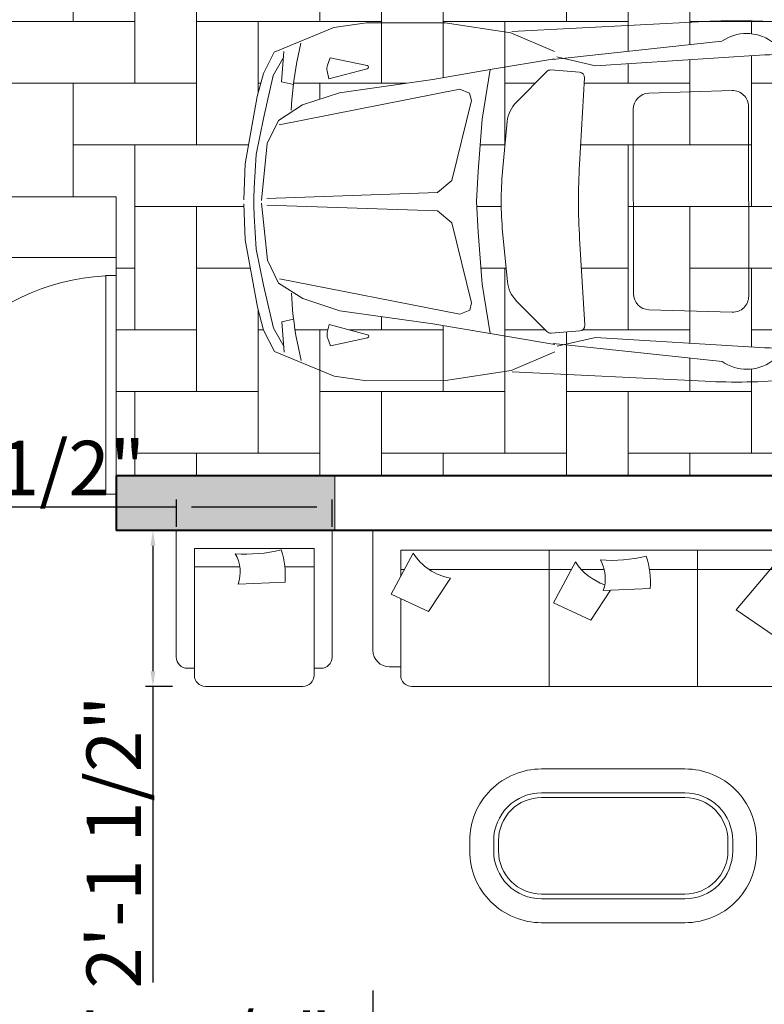
# Model space of a CAD drawing. Units: inches. Extents: x 2337 to 3570, y 1258 to 1938.
# Tile 13 of 30: x 2704 to 2827, y 1677 to 1839. Entities that reach past the tile are written whole.
import ezdxf

# ---------------------------------------------------------------- set-up
doc = ezdxf.new("R2010")
doc.units = ezdxf.units.IN
for name, color, linetype, lineweight in [('A-ANNO-DIMS', 2, 'Continuous', 18), ('A-DOOR', 4, 'Continuous', 20), ('A-FLOR-PATT', 252, 'Continuous', 13), ('A-FLOR-STRS', 7, 'Continuous', 20), ('A-GLAZ', 4, 'Continuous', 18), ('A-WALL', 7, 'Continuous', 40), ('furn', 8, 'Continuous', 18), ('L-SITE-VEHI', 8, 'Continuous', 18)]:
    doc.layers.add(name, color=color, linetype=linetype, lineweight=lineweight)
doc.layers.add('A-WALL-PATT', color=18, linetype='Continuous', lineweight=13, true_color=0x000000)
doc.styles.get("Standard").update_dxf_attribs({"font": 'arial.ttf'})
doc.dimstyles.new('ISO-25', dxfattribs={"dimtxt": 9, "dimasz": 2.5, "dimexe": 1.25, "dimexo": 0.625, "dimtad": 1, "dimdec": 1, "dimlunit": 3, "dimtxsty": 'Standard', "dimcen": 2.5, "dimadec": 0, "dimazin": 0, "dimtfac": 1, "dimtdec": 1, "dimtmove": 0, "dimatfit": 3, "dimfxl": 1, "dimarcsym": 0})

# ---------------------------------------------------------------- blocks, each defined once
blk = doc.blocks.new('*U2')
for p, q in [((0, 0), (0, -6)), ((36, 0), (36, -6))]:
    blk.add_line(p, q)
blk.add_lwpolyline([(0, 0), (0, 36), (1.75, 36), (1.75, 0)], close=True)
blk.add_arc((0, 0), 36, 0, 90)
blk = doc.blocks.new('sofa-11')
at = {"color": 0, "linetype": 'ByBlock'}
for p, q in [((0, 2.05), (0.55, 2.05)), ((0, 0), (0, 2.05)), ((0.3008, 2.0175), (0.1161, 1.919)), ((0.3779, 1.85), (0.3008, 2.0175)), ((0.6, 2), (0.6, 1.95)), ((0.1, 1.95), (0.1743, 1.95)), ((0.1, 0.0875), (0.1, 1.95)), ((0.3319, 1.95), (0.65, 1.95)), ((0.7, 1.9), (0.7, 0.3768)), ((0.2, 0.8184), (0.2, 1.8305)), ((0.2281, 1.7514), (0.3779, 1.85)), ((0.1, 1.3), (0.7, 1.3)), ((0.2865, 0.8646), (0.1018, 0.766)), ((0.3637, 0.697), (0.2865, 0.8646)), ((0.2138, 0.5985), (0.3637, 0.697)), ((0.3623, 0.7), (2.6, 0.7)), ((1.3167, 0.7), (1.3167, 0.0875)), ((1.9833, 0.7), (1.9833, 0.0875)), ((0.2, 0.175), (0.2, 0.6475)), ((2.65, 0.65), (2.65, 0.6125)), ((2.65, 0.3062), (2.65, 0.6125)), ((2.65, 0.6125), (2.7, 0.6125)), ((2.775, 0.5375), (2.775, 0)), ((1.1431, 0.3556), (0.9718, 0.4727)), ((0.7655, 0.4423), (0.6064, 0.2832)), ((0.8605, 0.3474), (0.7655, 0.4423)), ((1.707, 0.2682), (1.7953, 0.4025)), ((1.7953, 0.4025), (1.9629, 0.3253)), ((0.9718, 0.1545), (1.1431, 0.3556)), ((2.4266, 0.2138), (2.5252, 0.3637)), ((2.5252, 0.3637), (2.6927, 0.2865)), ((1.9629, 0.3253), (1.8643, 0.1406)), ((0.6064, 0.2832), (0.7655, 0.1241)), ((1.5293, 0.2606), (1.7399, 0.2695)), ((2.6927, 0.2865), (2.5942, 0.1018)), ((0.7655, 0.1241), (0.9027, 0.2613)), ((2.65, 0.0875), (2.65, 0.2065)), ((0.7147, 0.175), (0.2, 0.175)), ((1.5323, 0.175), (0.8164, 0.175)), ((1.8381, 0.175), (1.7356, 0.175)), ((2.5231, 0.175), (1.8827, 0.175)), ((2.65, 0.175), (2.6332, 0.175)), ((0.1, 0.0875), (2.65, 0.0875)), ((2.775, 0), (0, 0))]:
    blk.add_line(p, q, dxfattribs=at)
for centre, radius, start, end in [((0.55, 2), 0.05, 0, 90), ((0.65, 1.9), 0.05, 0, 90), ((-0.0168, 1.709), 0.2485, 9.843, 57.6699), ((-0.0311, 0.556), 0.2485, 9.843, 57.6699), ((2.6, 0.65), 0.05, 360, 90), ((2.7, 0.5375), 0.075, 0, 90), ((0.5496, 0.7358), 0.4975, 301.9301, 328.0699), ((0.7356, 0.0774), 0.2485, 18.0785, 71.9215), ((1.8968, 0.215), 0.1661, 160.8325, 209.9235), ((1.902, 0.2307), 0.3739, 175.4155, 198.0697), ((1.6543, 0.0077), 0.2485, 32.3301, 71.5057), ((2.3841, -0.0311), 0.2485, 32.3301, 80.157), ((1.7033, -0.512), 0.6461, 85.599, 104.0402)]:
    blk.add_arc(centre, radius, start, end, dxfattribs=at)
blk = doc.blocks.new('sofa-15')
at = {"color": 0, "linetype": 'ByBlock'}
for p, q in [((0.1312, 0.7), (0.5687, 0.7)), ((0.0812, 0.0812), (0.0812, 0.65)), ((0.6187, 0.65), (0.6187, 0.6187)), ((0.05, 0.6187), (0.0812, 0.6187)), ((0.65, 0.6187), (0.6187, 0.6187)), ((0.6187, 0.6187), (0.6187, 0.0812)), ((0, 0.5687), (0, 0)), ((0.7, 0), (0.7, 0.5687)), ((0.2114, 0.2325), (0.4221, 0.2414)), ((0.0812, 0.1625), (0.2124, 0.1625)), ((0.4147, 0.1625), (0.6187, 0.1625)), ((0.6187, 0.0812), (0.0812, 0.0812)), ((0, 0), (0.7, 0))]:
    blk.add_line(p, q, dxfattribs=at)
for centre, radius, start, end in [((0.1312, 0.65), 0.05, 90, 180), ((0.5687, 0.65), 0.05, 0, 90), ((0.05, 0.5687), 0.05, 90, 180), ((0.65, 0.5687), 0.05, 360, 90), ((0.5841, 0.2026), 0.3739, 175.4155, 198.0697), ((0.5789, 0.1869), 0.1661, 160.8325, 209.9235), ((0.3854, -0.5401), 0.6461, 85.599, 104.0402)]:
    blk.add_arc(centre, radius, start, end, dxfattribs=at)
blk = doc.blocks.new('A$C4A3239E3')
for p, q in [((1.2507, 1.6335), (2.1522, 1.6799)), ((2.5445, 1.6742), (3.2816, 1.6148)), ((0.2661, 1.5794), (0.2592, 1.5495)), ((1.4425, 1.5023), (2.2313, 1.5881)), ((2.4629, 1.587), (3.3117, 1.4863)), ((2.7875, 1.5463), (3.0567, 1.5859)), ((3.4104, 1.6024), (3.6491, 1.5899)), ((0.1752, 1.399), (0.1867, 1.5408)), ((1.6407, 1.4739), (2.4076, 1.5225)), ((2.597, 1.5244), (3.3012, 1.4943)), ((3.8218, 1.5205), (3.7519, 1.525)), ((3.7813, 1.5317), (3.8128, 1.5185)), ((0.1359, 1.4288), (0.1867, 1.515)), ((0.3898, 1.477), (0.4021, 1.5106)), ((0.4021, 1.5106), (0.5754, 1.4741)), ((1.4497, 1.5063), (1.149, 1.4553)), ((1.4612, 1.5146), (1.6407, 1.4739)), ((3.3012, 1.4943), (3.4322, 1.4598)), ((3.8334, 1.3629), (3.8334, 1.5081)), ((3.8376, 1.5081), (3.8668, 1.4958)), ((0.0905, 1.2265), (0.1359, 1.4288)), ((0.3963, 1.4117), (0.388, 1.4492)), ((0.5758, 1.4596), (0.3963, 1.4117)), ((1.2717, 1.3033), (1.4134, 1.4465)), ((1.4329, 1.4538), (1.567, 1.4437)), ((0.2308, 1.3867), (0.1752, 1.399)), ((1.59, 1.4175), (1.5668, 1.0125)), ((1.8899, 1.3452), (2.2788, 1.3576)), ((3.6217, 1.372), (3.7108, 1.3099)), ((3.7558, 1.3393), (3.8231, 1.3506)), ((3.8137, 1.3503), (3.8686, 1.2144)), ((0.224, 1.314), (0.2207, 1.2655)), ((3.4158, 1.3024), (3.4294, 1.0516)), ((3.4434, 1.3284), (3.584, 1.3121)), ((1.8186, 0.4085), (1.8178, 1.2708)), ((2.3557, 1.283), (2.3566, 0.3973)), ((3.7535, 1.2644), (3.8014, 1.2553)), ((3.8014, 1.2553), (3.8941, 1.199)), ((0.0565, 1.0588), (0.0905, 1.2265)), ((1.2074, 0.9801), (1.2293, 1.2125)), ((3.6693, 1.236), (3.7299, 0.9762)), ((3.7713, 1.2181), (3.8245, 0.9626)), ((3.8941, 1.199), (3.9452, 0.89)), ((0.0481, 0.9038), (0.0565, 1.0588)), ((3.4294, 1.0516), (3.4292, 0.8428)), ((3.9292, 0.9941), (3.9933, 0.9668)), ((3.9933, 0.9668), (4.0172, 0.906)), ((4.0172, 0.906), (4.0211, 0.842)), ((3.4299, 0.6309), (3.4292, 0.8396)), ((4.0174, 0.7775), (4.0211, 0.8416)), ((3.8948, 0.4844), (3.9453, 0.7934)), ((0.0482, 0.7723), (0.0569, 0.6172)), ((3.9936, 0.7167), (4.0174, 0.7775)), ((1.2077, 0.6979), (1.23, 0.4656)), ((3.6701, 0.4469), (3.7301, 0.7068)), ((3.772, 0.465), (3.8248, 0.7206)), ((3.9295, 0.6893), (3.9936, 0.7167)), ((1.5911, 0.2613), (1.5671, 0.6662)), ((0.0569, 0.6172), (0.0912, 0.4496)), ((3.4167, 0.38), (3.4299, 0.6309)), ((3.8022, 0.4279), (3.8948, 0.4844)), ((3.8147, 0.3328), (3.8693, 0.4688)), ((0.0912, 0.4496), (0.1371, 0.2474)), ((3.7543, 0.4187), (3.8022, 0.4279)), ((0.2249, 0.3624), (0.2215, 0.4109)), ((1.2726, 0.3749), (1.4146, 0.232)), ((3.4444, 0.354), (3.585, 0.3707)), ((3.6228, 0.3107), (3.7117, 0.3731)), ((1.8909, 0.3342), (2.2798, 0.3226)), ((3.7568, 0.3438), (3.8241, 0.3326)), ((0.2318, 0.2897), (0.1763, 0.2773)), ((0.1763, 0.2773), (0.1881, 0.1355)), ((3.8345, 0.3203), (3.8347, 0.1751)), ((0.1371, 0.2474), (0.188, 0.1613)), ((0.3975, 0.2651), (0.3892, 0.2275)), ((0.5771, 0.2174), (0.3975, 0.2651)), ((1.4341, 0.2247), (1.5682, 0.235)), ((0.3911, 0.1998), (0.4034, 0.1661)), ((0.4034, 0.1661), (0.5767, 0.203)), ((1.451, 0.1722), (1.1502, 0.2226)), ((1.4625, 0.1639), (1.6419, 0.205)), ((1.6419, 0.205), (2.4089, 0.1579)), ((2.4644, 0.0936), (3.313, 0.1959)), ((2.5984, 0.1564), (3.3024, 0.1879)), ((3.3024, 0.1879), (3.4334, 0.2226)), ((3.8389, 0.1752), (3.8681, 0.1875)), ((1.4438, 0.1762), (2.2328, 0.0919)), ((3.8231, 0.1627), (3.7532, 0.1581)), ((3.7826, 0.1514), (3.8141, 0.1647)), ((0.2676, 0.0971), (0.2606, 0.127)), ((2.7889, 0.1349), (3.0581, 0.0958)), ((3.4119, 0.0799), (3.6506, 0.0929)), ((2.5461, 0.0065), (3.2831, 0.0673)), ((1.2522, 0.0446), (2.1538, 0))]:
    blk.add_line(p, q)
for points in [[(0, 0.8478), (0.0053, 1.0159), (0.0622, 1.3298), (0.0905, 1.4375), (0.1412, 1.5365), (0.4188, 1.6529), (0.572, 1.6743), (0.9399, 1.6743), (1.2458, 1.627), (1.4497, 1.5408)], [(0.0815, 0.8439), (0.1088, 1.11), (0.1609, 1.2182), (0.2737, 1.2906), (0.4463, 1.3472), (0.8811, 1.4091), (1.149, 1.4553), (1.1121, 1.224), (1.0933, 0.9813), (1.085, 0.8389)], [(0.1644, 1.198), (1.0072, 1.3636), (1.0537, 1.3462), (1.0619, 1.3117), (0.9706, 0.937), (0.9035, 0.8818), (0.106, 0.853)], [(0, 0.8281), (0.0056, 0.6601), (0.0632, 0.3462), (0.0916, 0.2386), (0.1426, 0.1398), (0.4204, 0.0239), (0.5737, 0.0028), (0.9415, 0.0032), (1.2473, 0.0511), (1.4511, 0.1377)], [(0.0815, 0.8322), (0.1094, 0.5662), (0.1616, 0.4581), (0.2746, 0.3859), (0.4473, 0.3296), (0.8822, 0.2683), (1.1502, 0.2226), (1.1128, 0.4539), (1.0936, 0.6965), (1.085, 0.8389)], [(0.1651, 0.4782), (1.0082, 0.314), (1.0547, 0.3316), (1.0628, 0.366), (0.9708, 0.7406), (0.9036, 0.7957), (0.1061, 0.8232)]]:
    blk.add_lwpolyline(points)
for centre, radius, start, end in [((2.3053, -1.296), 2.9798, 85.3952, 92.9452), ((2.3463, 1.4226), 0.2016, 54.6492, 124.7769), ((3.3168, -0.183), 1.7879, 86.9998, 98.3676), ((3.6355, 1.3122), 0.278, 57.3299, 87.1824), ((1.7104, 1.2122), 1.4899, 166.9166, 176.0811), ((2.5206, -0.2618), 1.7879, 87.5491, 93.6237), ((4.0973, 1.4394), 0.3558, 166.0961, 196.3535), ((3.821, 1.5081), 0.0124, 0, 86.3304), ((0.4365, 1.46), 0.0497, 159.9787, 192.5384), ((0.5739, 1.4668), 0.00745, 284.96, 78.1125), ((3.2466, 0.8963), 0.8285, 356.2451, 44.5195), ((3.8091, 1.3584), 0.149, 46.3836, 67.2014), ((1.431, 1.429), 0.0248, 85.7151, 135.3046), ((1.5652, 1.4189), 0.0248, 356.7256, 85.7151), ((3.2805, 0.8834), 0.596, 55.07, 75.2551), ((3.6181, 1.158), 0.4258, 30.4577, 46.3836), ((1.8923, 1.2708), 0.0745, 91.8201, 179.9989), ((2.2812, 1.2831), 0.0745, 359.9245, 91.8201), ((3.821, 1.3629), 0.0124, 279.6077, 0), ((3.1325, 0.8724), 0.9892, 358.0694, 30.4577), ((1.3776, 1.1985), 0.149, 135.3046, 174.6214), ((3.4406, 1.3037), 0.0248, 83.376, 183.115), ((3.5726, 1.2134), 0.0993, 13.1226, 83.376), ((3.6254, 1.1877), 0.149, 11.7694, 55.07), ((4.5417, 0.8423), 2.9798, 176.7256, 183.3874), ((2.6908, 0.8405), 1.4899, 174.6214, 185.4916), ((3.1495, 0.8409), 0.596, 346.9903, 13.1226), ((3.2411, 0.841), 0.596, 348.3436, 11.7694), ((1.2382, 0.8392), 1.1919, 176.8942, 183.2188), ((3.6512, 0.8414), 0.298, 350.7246, 9.3883), ((3.2467, 0.7858), 0.8285, 315.5935, 3.8679), ((3.1326, 0.8094), 0.9892, 329.6553, 2.0435), ((1.3783, 0.4799), 0.149, 185.4916, 224.8083), ((3.6261, 0.4951), 0.149, 305.0429, 348.3436), ((3.5733, 0.4693), 0.0993, 276.737, 346.9903), ((1.8931, 0.4086), 0.0745, 180.1141, 268.2929), ((2.2821, 0.397), 0.0745, 268.2929, 0.1885), ((3.4415, 0.3787), 0.0248, 176.9979, 276.737), ((1.7111, 0.4671), 1.4899, 184.0319, 193.1964), ((4.0985, 0.2443), 0.3558, 163.7595, 194.0169), ((3.822, 0.3203), 0.0124, 0.113, 80.5053), ((3.2806, 0.7987), 0.596, 284.8579, 305.0429), ((3.6188, 0.5248), 0.4258, 313.7293, 329.6553), ((1.4322, 0.2495), 0.0248, 224.8083, 274.3979), ((1.5663, 0.2598), 0.0248, 274.3979, 3.3874), ((0.4377, 0.2169), 0.0497, 167.5746, 200.1342), ((0.5752, 0.2102), 0.00745, 282.0005, 75.153), ((3.8101, 0.3247), 0.149, 292.9116, 313.7293), ((2.5184, 1.9425), 1.7879, 266.4893, 272.5638), ((3.8223, 0.1751), 0.0124, 273.7825, 0.113), ((2.3474, 0.2577), 0.2016, 235.336, 305.4638), ((3.3148, 1.8652), 1.7879, 261.7454, 273.1132), ((3.6364, 0.3706), 0.278, 272.9306, 302.783), ((2.3011, 2.9762), 2.9798, 267.1678, 274.7177)]:
    blk.add_arc(centre, radius, start, end)
blk = doc.blocks.new('*D86')
at = {"layer": 'A-ANNO-DIMS', "color": 0, "lineweight": -2, "transparency": 16777216}
for p, q in [((2762.09, 1679.33), (2762.09, 1663.44)), ((2863.84, 1679.33), (2863.84, 1663.44)), ((2762.09, 1664.69), (2617.85, 1664.69)), ((2861.34, 1664.69), (2764.59, 1664.69))]:
    blk.add_line(p, q, dxfattribs=at)
at = {"layer": 'A-ANNO-DIMS', "color": 0, "transparency": 16777216}
for points in [[(2764.59, 1665.11), (2764.59, 1664.28), (2762.09, 1664.69)], [(2861.34, 1665.11), (2861.34, 1664.28), (2863.84, 1664.69)]]:
    blk.add_solid(points, dxfattribs=at)
at = {"layer": 'Defpoints', "color": 0, "transparency": 16777216}
for p in [(2762.09, 1679.95), (2863.84, 1679.95), (2762.09, 1664.69)]:
    blk.add_point(p, dxfattribs=at)
at = {"layer": 'A-ANNO-DIMS', "color": 0, "transparency": 16777216, "insert": (2688.72, 1669.97), "char_height": 9, "attachment_point": 5}
blk.add_mtext('CORNER SOFA 8\'-5 1/2"', dxfattribs=at)
blk = doc.blocks.new('*D88')
at = {"layer": 'A-ANNO-DIMS', "color": 0, "lineweight": -2, "transparency": 16777216}
for p, q in [((2729.73, 1755.74), (2729.73, 1760.22)), ((2755.39, 1755.74), (2755.39, 1760.22)), ((2729.73, 1758.97), (2610.01, 1758.97)), ((2752.89, 1758.97), (2732.23, 1758.97))]:
    blk.add_line(p, q, dxfattribs=at)
at = {"layer": 'A-ANNO-DIMS', "color": 0, "transparency": 16777216}
for points in [[(2732.23, 1759.38), (2732.23, 1758.55), (2729.73, 1758.97)], [(2752.89, 1759.38), (2752.89, 1758.55), (2755.39, 1758.97)]]:
    blk.add_solid(points, dxfattribs=at)
at = {"layer": 'Defpoints', "color": 0, "transparency": 16777216}
for p in [(2729.73, 1758.97), (2729.73, 1755.12), (2755.39, 1755.12)]:
    blk.add_point(p, dxfattribs=at)
at = {"layer": 'A-ANNO-DIMS', "color": 0, "transparency": 16777216, "insert": (2668.62, 1764.24), "char_height": 9, "attachment_point": 5}
blk.add_mtext('ARMCHAIR 2\'-1 1/2"', dxfattribs=at)
blk = doc.blocks.new('*D89')
at = {"layer": 'A-ANNO-DIMS', "color": 0, "lineweight": -2, "transparency": 16777216}
for p, q in [((2729.1, 1755.12), (2724.63, 1755.12)), ((2725.88, 1752.62), (2725.88, 1731.95)), ((2729.1, 1729.45), (2724.63, 1729.45)), ((2725.88, 1729.45), (2725.88, 1680.65))]:
    blk.add_line(p, q, dxfattribs=at)
at = {"layer": 'A-ANNO-DIMS', "color": 0, "transparency": 16777216}
for points in [[(2725.46, 1752.62), (2726.29, 1752.62), (2725.88, 1755.12)], [(2725.46, 1731.95), (2726.29, 1731.95), (2725.88, 1729.45)]]:
    blk.add_solid(points, dxfattribs=at)
at = {"layer": 'Defpoints', "color": 0, "transparency": 16777216}
for p in [(2729.73, 1755.12), (2725.88, 1729.45), (2729.73, 1729.45)]:
    blk.add_point(p, dxfattribs=at)
at = {"layer": 'A-ANNO-DIMS', "color": 0, "transparency": 16777216, "insert": (2720.6, 1703.8), "char_height": 9, "attachment_point": 5, "rotation": 90}
blk.add_mtext('2\'-1 1/2"', dxfattribs=at)

msp = doc.modelspace()

# ---------------------------------------------------------------- hatches: boundary and pattern name
at = {"layer": 'A-FLOR-PATT', "transparency": 33554687}
h = msp.add_hatch(dxfattribs=at)
h.set_pattern_fill('AR-HBONE', color=256, scale=0.1, angle=45)
h.paths.add_polyline_path([(2902.84, 1875.12), (2899.84, 1875.12), (2899.84, 1887.12), (2671.84, 1887.12), (2671.84, 1857.12), (2681.84, 1857.12), (2681.84, 1810.12), (2719.84, 1810.12), (2719.84, 1764.12), (2872.84, 1764.12), (2899.84, 1764.12), (2899.84, 1779.12), (2902.84, 1779.12)])
h.paths.add_polyline_path([(2854.18, 1832.56), (2857.32, 1832.42), (2861.94, 1831.21, -0.088302), (2868.63, 1828.11), (2871.77, 1825.92, -0.105467), (2873.27, 1824.31), (2874.97, 1823.99), (2877.34, 1822.55), (2875.42, 1827.3), (2873.36, 1826.95, -0.132795), (2873.22, 1833.51), (2876.1, 1833.32), (2876.1, 1832.97), (2877.28, 1832.48, -0.091085), (2878.86, 1831.44, -0.069602), (2881.45, 1828.18, -0.141553), (2886.25, 1809.41, -0.141553), (2881.49, 1790.63, -0.069602), (2878.91, 1787.37, -0.091085), (2877.32, 1786.33), (2876.14, 1785.83, -0.354729), (2875.73, 1785.45), (2873.27, 1785.29, -0.132795), (2873.39, 1791.84), (2875.45, 1791.49), (2877.36, 1796.25), (2874.99, 1794.81), (2873.3, 1794.48, -0.105467), (2871.8, 1792.87), (2868.67, 1790.67, -0.088302), (2861.99, 1787.56), (2857.37, 1786.34), (2854.23, 1786.2), (2827.8, 1783.01, -0.315912), (2819.63, 1782.95), (2793.54, 1785.74), (2798.79, 1786.94), (2825.85, 1785.28, 0.026512), (2832.53, 1785.23), (2857.37, 1786.34), (2861.99, 1787.56, 0.088302), (2868.67, 1790.67), (2871.8, 1792.87, 0.191215), (2873.93, 1796.11), (2875.79, 1805.13, 0.102572), (2875.78, 1813.67), (2873.91, 1822.68, 0.191215), (2871.77, 1825.92), (2868.63, 1828.11, 0.088302), (2861.94, 1831.21), (2857.32, 1832.42), (2832.48, 1833.49, 0.026512), (2825.8, 1833.42), (2798.75, 1831.7), (2793.5, 1832.9), (2819.58, 1835.73, -0.315912), (2827.75, 1835.69)], flags=16)
h.paths.add_polyline_path([(2862.34, 1826.57), (2867.3, 1826, -0.316515), (2870.31, 1823.31), (2872.44, 1814.15, -0.11452), (2872.45, 1804.64), (2870.34, 1795.48, -0.316515), (2867.33, 1792.79), (2862.37, 1792.2, -0.464922), (2861.4, 1793.12), (2861.86, 1801.97), (2861.84, 1809.39), (2861.85, 1816.81), (2861.36, 1825.65, -0.464922)], flags=16)
h.paths.add_polyline_path([(2821.29, 1791.09), (2807.57, 1791.5, -0.405226), (2805.02, 1794.12), (2805.02, 1794.12, 0.40508), (2807.57, 1791.5), (2821.29, 1791.09, 0.423258), (2824, 1793.72), (2824, 1793.72, -0.423258)], flags=16)
h.paths.add_polyline_path([(2879.43, 1814.8), (2881.74, 1813.82), (2882.58, 1811.67), (2882.72, 1809.41), (2882.59, 1807.14), (2881.75, 1804.99), (2879.44, 1804.01), (2880.04, 1807.7, 0.081616), (2880.04, 1811.11)], flags=0)
h.paths.add_polyline_path([(2796.96, 1829.72), (2796.14, 1815.43, 0.029076), (2796.15, 1803.21), (2797, 1788.93, -0.409057), (2796.19, 1788), (2791.05, 1787.61), (2785.76, 1792.94, -0.173254), (2784.26, 1796.14), (2783.47, 1804.33, -0.047466), (2783.46, 1814.29), (2784.23, 1822.48, -0.173254), (2785.73, 1825.69), (2791.01, 1831.02), (2796.15, 1830.64, -0.409057)], flags=16)
h.paths.add_polyline_path([(2750.34, 1835.79), (2750.01, 1834.37, 0.040009), (2748.77, 1826.06), (2748.63, 1824.02), (2750.53, 1825.24), (2756.61, 1827.24), (2771.95, 1829.42), (2781.4, 1831.05), (2780.1, 1822.89), (2779.44, 1814.33), (2779.14, 1809.3), (2779.45, 1804.28), (2780.13, 1795.72), (2781.44, 1787.56), (2771.99, 1789.17), (2756.65, 1791.34), (2750.56, 1793.32), (2748.66, 1794.54), (2748.8, 1792.49, 0.040009), (2750.06, 1784.19), (2750.4, 1782.77), (2745.9, 1784.64), (2744.1, 1788.13), (2743.1, 1791.92), (2741.07, 1803), (2740.86, 1809.27), (2741.06, 1815.55), (2743.06, 1826.62), (2744.06, 1830.42), (2745.85, 1833.91)], flags=16)
h.paths.add_polyline_path([(2761.18, 1831.2), (2754.85, 1829.51), (2754.56, 1830.83, -0.143032), (2754.62, 1831.81), (2755.05, 1833), (2761.17, 1831.71, -0.789416)], flags=16)
h.paths.add_polyline_path([(2761.23, 1787.38), (2754.89, 1789.06), (2754.6, 1787.74, 0.143032), (2754.66, 1786.76), (2755.1, 1785.57), (2761.21, 1786.87, 0.789416)], flags=16)
h.paths.add_polyline_path([(2689.03, 1816.17), (2701.27, 1816.17), (2701.27, 1823.8), (2689.03, 1823.8)], flags=24)
h.paths.add_polyline_path([(2755.38, 1858.95), (2808.72, 1858.95), (2808.72, 1885.07), (2755.38, 1885.07)], flags=24)
at = {"layer": 'A-WALL-PATT'}
h = msp.add_hatch(color=256, dxfattribs=at)
h.dxf.hatch_style = 1
h.paths.add_polyline_path([(2671.84, 1857.12), (2455.84, 1857.12), (2455.84, 1824.12), (2464.84, 1824.12), (2464.84, 1848.12), (2671.84, 1848.12)])
h.paths.add_polyline_path([(2566.84, 1764.12), (2464.84, 1764.12), (2464.84, 1788.12), (2455.84, 1788.12), (2455.84, 1743.12), (2464.84, 1743.12), (2464.84, 1755.12), (2566.84, 1755.12)])
h.paths.add_polyline_path([(2683.84, 1761.12), (2683.84, 1764.12), (2602.84, 1764.12), (2602.84, 1755.12), (2608.84, 1755.12), (2608.84, 1701.12), (2662.84, 1701.12), (2662.84, 1605.12), (2671.84, 1605.12), (2671.84, 1713.12), (2662.84, 1713.12), (2662.84, 1707.12), (2614.84, 1707.12), (2614.84, 1755.12), (2662.84, 1755.12), (2662.84, 1749.12), (2671.84, 1749.12), (2671.84, 1755.12), (2683.84, 1755.12)])
h.paths.add_polyline_path([(2464.84, 1707.12), (2455.84, 1707.12), (2455.84, 1617.12), (2464.84, 1617.12), (2464.84, 1635.12), (2506.84, 1635.12), (2506.84, 1641.12), (2464.84, 1641.12)])
h.paths.add_polyline_path([(2542.84, 1551.12), (2464.84, 1551.12), (2464.84, 1569.12), (2455.84, 1569.12), (2455.84, 1518.12), (2464.84, 1518.12), (2464.84, 1542.12), (2542.84, 1542.12)])
h.paths.add_polyline_path([(2464.84, 1482.12), (2455.84, 1482.12), (2455.84, 1410.12), (2464.84, 1410.12)])
h.paths.add_polyline_path([(2626.84, 1350.12), (2590.84, 1350.12), (2590.84, 1380.12), (2584.84, 1380.12), (2584.84, 1350.12), (2464.84, 1350.12), (2464.84, 1374.12), (2455.84, 1374.12), (2455.84, 1341.12), (2626.84, 1341.12)])
h.paths.add_polyline_path([(2662.84, 1416.12), (2686.84, 1416.12), (2686.84, 1422.12), (2590.84, 1422.12), (2590.84, 1542.12), (2680.84, 1542.12), (2680.84, 1551.12), (2671.84, 1551.12), (2671.84, 1557.12), (2662.84, 1557.12), (2662.84, 1551.12), (2578.84, 1551.12), (2578.84, 1542.12), (2584.84, 1542.12), (2584.84, 1410.12), (2590.84, 1410.12), (2590.84, 1416.12), (2656.84, 1416.12), (2656.84, 1350.12), (2650.84, 1350.12), (2650.84, 1341.12), (2731.84, 1341.12), (2731.84, 1362.12), (2722.84, 1362.12), (2722.84, 1350.12), (2662.84, 1350.12)])
h.paths.add_polyline_path([(2731.84, 1434.12), (2722.84, 1434.12), (2722.84, 1422.12), (2716.84, 1422.12), (2716.84, 1416.12), (2722.84, 1416.12), (2722.84, 1386.12), (2731.84, 1386.12)], flags=17)
h.paths.add_polyline_path([(2731.84, 1542.12), (2752.84, 1542.12), (2752.84, 1551.12), (2716.84, 1551.12), (2716.84, 1545.12), (2716.84, 1542.12), (2722.84, 1542.12), (2722.84, 1482.12), (2731.84, 1482.12)])
h.paths.add_polyline_path([(2809.84, 1551.12), (2788.84, 1551.12), (2788.84, 1542.12), (2809.84, 1542.12), (2809.84, 1548.12)])
h.paths.add_polyline_path([(2872.84, 1647.12), (2863.84, 1647.12), (2863.84, 1551.12), (2857.84, 1551.12), (2857.84, 1548.12), (2857.84, 1542.12), (2872.84, 1542.12)])
h.paths.add_polyline_path([(2872.84, 1764.12), (2827.84, 1764.12), (2827.84, 1755.12), (2863.84, 1755.12), (2863.84, 1719.12), (2872.84, 1719.12)])
h.paths.add_polyline_path([(2755.84, 1764.12), (2719.84, 1764.12), (2719.84, 1755.12), (2755.84, 1755.12)])

# ---------------------------------------------------------------- linework, layer by layer
at = {"layer": 'A-FLOR-STRS'}
for p, q in [((2719.84, 1810.12), (2681.84, 1810.12)), ((2719.84, 1764.12), (2719.84, 1810.12)), ((2719.84, 1800.12), (2671.84, 1800.12))]:
    msp.add_line(p, q, dxfattribs=at)
at = {"layer": 'A-GLAZ'}
msp.add_line((2755.84, 1764.12), (2755.84, 1755.12), dxfattribs=at)
at = {"layer": 'A-WALL'}
for p, q in [((2872.84, 1764.12), (2719.84, 1764.12)), ((2719.84, 1764.12), (2719.84, 1755.12)), ((2863.84, 1755.12), (2719.84, 1755.12))]:
    msp.add_line(p, q, dxfattribs=at)
at = {"layer": 'furn'}
for points in [[(2813.5, 1690.51), (2789.88, 1690.51, -0.414214), (2778.06, 1702.32), (2778.06, 1704.04, -0.414214), (2789.88, 1715.85), (2813.5, 1715.85, -0.414214), (2825.31, 1704.04), (2825.31, 1702.32, -0.414214)], [(2813.5, 1694.45), (2789.88, 1694.45, -0.414214), (2782, 1702.32), (2782, 1704.04, -0.414214), (2789.88, 1711.91), (2813.5, 1711.91, -0.414214), (2821.37, 1704.04), (2821.37, 1702.32, -0.414214)], [(2813.5, 1695.24), (2789.88, 1695.24, -0.414214), (2782.79, 1702.32), (2782.79, 1704.04, -0.414214), (2789.88, 1711.13), (2813.5, 1711.13, -0.414214), (2820.58, 1704.04), (2820.58, 1702.32, -0.414214)]]:
    msp.add_lwpolyline(points, format="xyb", close=True, dxfattribs=at)

# ---------------------------------------------------------------- block references
at = {"layer": 'A-DOOR', "xscale": -1}
msp.add_blockref('*U2', (2719.84, 1761.12), dxfattribs=at)
at = {"layer": 'furn', "xscale": 36.66436083614781, "yscale": 36.66436083614781, "zscale": 36.66436083614781, "rotation": 180}
for name, p in [('sofa-15', (2755.39, 1755.12)), ('sofa-11', (2863.84, 1755.12))]:
    msp.add_blockref(name, p, dxfattribs=at)
at = {"layer": 'L-SITE-VEHI', "xscale": 35.27598425228, "yscale": 35.27598425228, "zscale": 35.27598425228}
msp.add_blockref('A$C4A3239E3', (2740.87, 1779.71), dxfattribs=at)

# ---------------------------------------------------------------- dimensions: what is measured, and where the dimension line sits
at = {"layer": 'A-ANNO-DIMS'}
for base, p1, p2, text, picture, middle in [((2729.73, 1758.97), (2755.39, 1755.12), (2729.73, 1755.12), 'ARMCHAIR <>', '*D88', (2668.62, 1764.24)), ((2762.0922, 1664.6925), (2863.8358, 1679.9541), (2762.0922, 1679.9541), 'CORNER SOFA <>', '*D86', (2688.7199, 1669.9741))]:
    dim = msp.add_linear_dim(base=base, p1=p1, p2=p2, angle=180, text=text, dimstyle='ISO-25', override={"dimdec": 1, "dimlfac": 1, "dimrnd": 0, "dimzin": 1, "dimdsep": 46, "dimlunit": 4, "dimfrac": 2}, dxfattribs=at)
    dim.commit()
    dim.dimension.update_dxf_attribs({"geometry": picture, "text_midpoint": middle})
dim = msp.add_linear_dim(base=(2725.88, 1729.45), p1=(2729.73, 1755.12), p2=(2729.73, 1729.45), angle=270, dimstyle='ISO-25', override={"dimdec": 1, "dimlfac": 1, "dimrnd": 0, "dimzin": 1, "dimdsep": 46, "dimlunit": 4, "dimfrac": 2}, dxfattribs=at)
dim.commit()
dim.dimension.update_dxf_attribs({"geometry": '*D89', "text_midpoint": (2720.6, 1703.8)})

doc.saveas('drawing.dxf')
